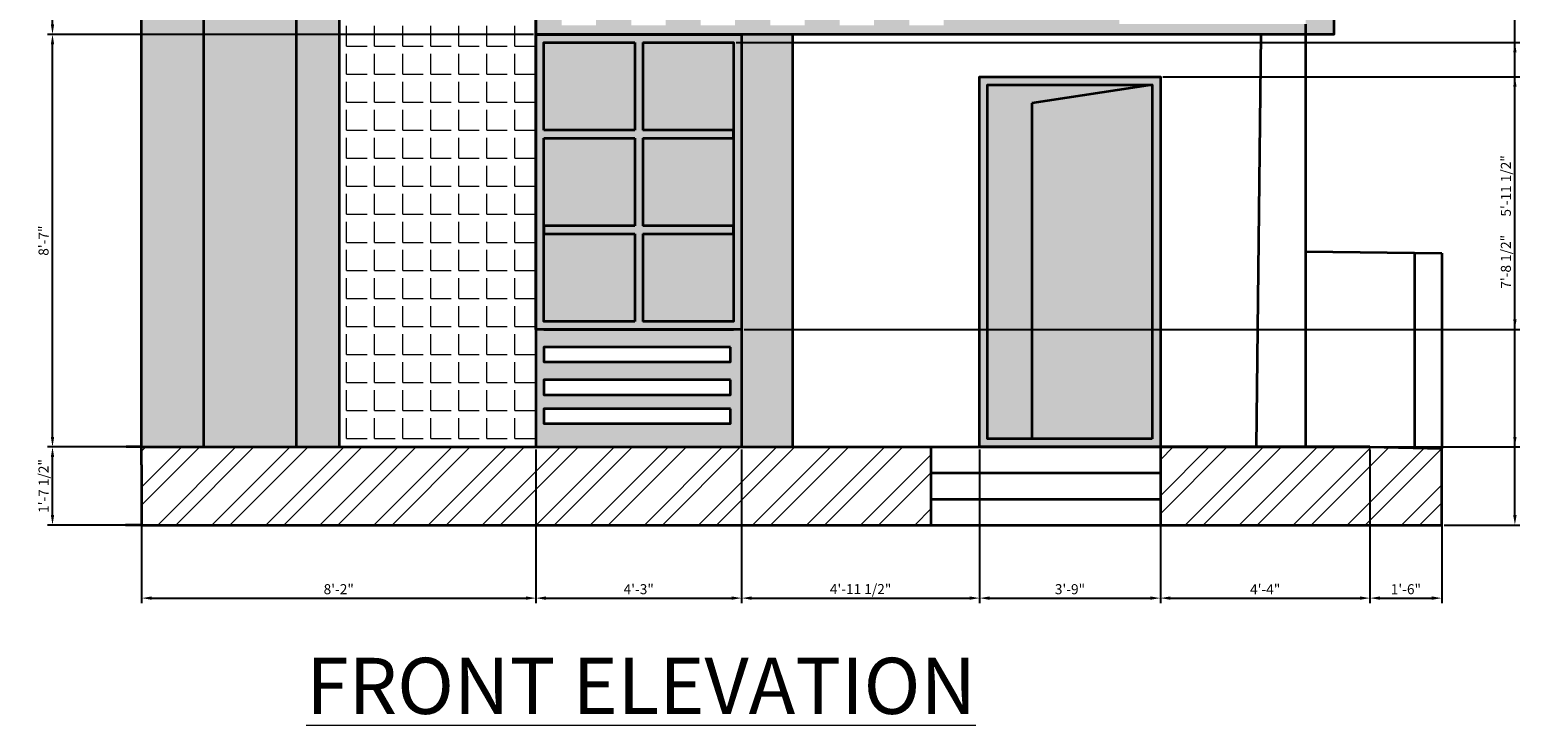
# Model space of a CAD drawing. Units: inches. Extents: x 2117 to 3047, y 1240 to 2266.
# Tile 2 of 4: x 2212 to 2584, y 1884 to 2058. Entities that reach past the tile are written whole.
import ezdxf

# ---------------------------------------------------------------- set-up
doc = ezdxf.new("R2010")
doc.units = ezdxf.units.IN
for name, color, linetype, lineweight in [('A-ANNO-DIMS', 2, 'Continuous', 18), ('A-ANNO-TEXT', 7, 'Continuous', 18), ('A-ELEV', 7, 'Continuous', 35), ('A-ELEV-PATT', 8, 'Continuous', 13)]:
    doc.layers.add(name, color=color, linetype=linetype, lineweight=lineweight)
doc.styles.get("Standard").update_dxf_attribs({"font": 'arial.ttf'})
doc.dimstyles.new('ISO-25', dxfattribs={"dimtxt": 2.5, "dimasz": 2.5, "dimexe": 1.25, "dimexo": 0.625, "dimtad": 1, "dimdec": 1, "dimlunit": 3, "dimtxsty": 'Standard', "dimcen": 2.5, "dimadec": 0, "dimazin": 0, "dimtfac": 1, "dimtdec": 1, "dimtmove": 0, "dimatfit": 3, "dimfxl": 1, "dimarcsym": 0})

# ---------------------------------------------------------------- blocks, each defined once
blk = doc.blocks.new('*D34')
at = {"layer": 'A-ANNO-DIMS', "color": 0, "lineweight": -2, "transparency": 16777216}
for p, q in [((2240.01, 1953.08), (2240.01, 1914.75)), ((2338.23, 1953.08), (2338.23, 1914.75)), ((2242.51, 1916), (2335.73, 1916))]:
    blk.add_line(p, q, dxfattribs=at)
at = {"layer": 'A-ANNO-DIMS', "color": 0, "transparency": 16777216}
for points in [[(2242.51, 1916.42), (2242.51, 1915.58), (2240.01, 1916)], [(2335.73, 1916.42), (2335.73, 1915.58), (2338.23, 1916)]]:
    blk.add_solid(points, dxfattribs=at)
at = {"layer": 'Defpoints', "color": 0, "transparency": 16777216}
for p in [(2240.01, 1953.7), (2338.23, 1953.7), (2338.23, 1916)]:
    blk.add_point(p, dxfattribs=at)
at = {"layer": 'A-ANNO-DIMS', "color": 0, "transparency": 16777216, "insert": (2289.12, 1917.9), "char_height": 2.5, "attachment_point": 5}
blk.add_mtext('8\'-2"', dxfattribs=at)
blk = doc.blocks.new('*D35')
at = {"layer": 'A-ANNO-DIMS', "color": 0, "lineweight": -2, "transparency": 16777216}
for p, q in [((2338.23, 1953.08), (2338.23, 1914.75)), ((2389.48, 1953.08), (2389.48, 1914.75)), ((2340.73, 1916), (2386.98, 1916))]:
    blk.add_line(p, q, dxfattribs=at)
at = {"layer": 'A-ANNO-DIMS', "color": 0, "transparency": 16777216}
for points in [[(2340.73, 1916.42), (2340.73, 1915.58), (2338.23, 1916)], [(2386.98, 1916.42), (2386.98, 1915.58), (2389.48, 1916)]]:
    blk.add_solid(points, dxfattribs=at)
at = {"layer": 'Defpoints', "color": 0, "transparency": 16777216}
for p in [(2338.23, 1953.7), (2389.48, 1953.7), (2389.48, 1916)]:
    blk.add_point(p, dxfattribs=at)
at = {"layer": 'A-ANNO-DIMS', "color": 0, "transparency": 16777216, "insert": (2363.85, 1917.9), "char_height": 2.5, "attachment_point": 5}
blk.add_mtext('4\'-3"', dxfattribs=at)
blk = doc.blocks.new('*D36')
at = {"layer": 'A-ANNO-DIMS', "color": 0, "lineweight": -2, "transparency": 16777216}
for p, q in [((2389.48, 1953.08), (2389.48, 1914.75)), ((2448.76, 1953.08), (2448.76, 1914.75)), ((2391.98, 1916), (2446.26, 1916))]:
    blk.add_line(p, q, dxfattribs=at)
at = {"layer": 'A-ANNO-DIMS', "color": 0, "transparency": 16777216}
for points in [[(2391.98, 1916.42), (2391.98, 1915.58), (2389.48, 1916)], [(2446.26, 1916.42), (2446.26, 1915.58), (2448.76, 1916)]]:
    blk.add_solid(points, dxfattribs=at)
at = {"layer": 'Defpoints', "color": 0, "transparency": 16777216}
for p in [(2389.48, 1953.7), (2448.76, 1953.7), (2448.76, 1916)]:
    blk.add_point(p, dxfattribs=at)
at = {"layer": 'A-ANNO-DIMS', "color": 0, "transparency": 16777216, "insert": (2419.12, 1917.92), "char_height": 2.5, "attachment_point": 5}
blk.add_mtext('4\'-11 1/2"', dxfattribs=at)
blk = doc.blocks.new('*D37')
at = {"layer": 'A-ANNO-DIMS', "color": 0, "lineweight": -2, "transparency": 16777216}
for p, q in [((2448.76, 1953.08), (2448.76, 1914.75)), ((2493.8, 1953.08), (2493.8, 1914.75)), ((2451.26, 1916), (2491.3, 1916))]:
    blk.add_line(p, q, dxfattribs=at)
at = {"layer": 'A-ANNO-DIMS', "color": 0, "transparency": 16777216}
for points in [[(2451.26, 1916.42), (2451.26, 1915.58), (2448.76, 1916)], [(2491.3, 1916.42), (2491.3, 1915.58), (2493.8, 1916)]]:
    blk.add_solid(points, dxfattribs=at)
at = {"layer": 'Defpoints', "color": 0, "transparency": 16777216}
for p in [(2448.76, 1953.7), (2493.8, 1953.7), (2493.8, 1916)]:
    blk.add_point(p, dxfattribs=at)
at = {"layer": 'A-ANNO-DIMS', "color": 0, "transparency": 16777216, "insert": (2471.28, 1917.9), "char_height": 2.5, "attachment_point": 5}
blk.add_mtext('3\'-9"', dxfattribs=at)
blk = doc.blocks.new('*D38')
at = {"layer": 'A-ANNO-DIMS', "color": 0, "lineweight": -2, "transparency": 16777216}
for p, q in [((2493.8, 1953.08), (2493.8, 1914.75)), ((2546.01, 1953.08), (2546.01, 1914.75)), ((2496.3, 1916), (2543.51, 1916))]:
    blk.add_line(p, q, dxfattribs=at)
at = {"layer": 'A-ANNO-DIMS', "color": 0, "transparency": 16777216}
for points in [[(2496.3, 1916.42), (2496.3, 1915.58), (2493.8, 1916)], [(2543.51, 1916.42), (2543.51, 1915.58), (2546.01, 1916)]]:
    blk.add_solid(points, dxfattribs=at)
at = {"layer": 'Defpoints', "color": 0, "transparency": 16777216}
for p in [(2493.8, 1953.7), (2546.01, 1953.7), (2546.01, 1916)]:
    blk.add_point(p, dxfattribs=at)
at = {"layer": 'A-ANNO-DIMS', "color": 0, "transparency": 16777216, "insert": (2519.91, 1917.88), "char_height": 2.5, "attachment_point": 5}
blk.add_mtext('4\'-4"', dxfattribs=at)
blk = doc.blocks.new('*D39')
at = {"layer": 'A-ANNO-DIMS', "color": 0, "lineweight": -2, "transparency": 16777216}
for p, q in [((2546.01, 1953.08), (2546.01, 1914.75)), ((2563.92, 1952.72), (2563.92, 1914.75)), ((2548.51, 1916), (2561.42, 1916))]:
    blk.add_line(p, q, dxfattribs=at)
at = {"layer": 'A-ANNO-DIMS', "color": 0, "transparency": 16777216}
for points in [[(2548.51, 1916.42), (2548.51, 1915.58), (2546.01, 1916)], [(2561.42, 1916.42), (2561.42, 1915.58), (2563.92, 1916)]]:
    blk.add_solid(points, dxfattribs=at)
at = {"layer": 'Defpoints', "color": 0, "transparency": 16777216}
for p in [(2546.01, 1953.7), (2563.92, 1953.34), (2563.92, 1916)]:
    blk.add_point(p, dxfattribs=at)
at = {"layer": 'A-ANNO-DIMS', "color": 0, "transparency": 16777216, "insert": (2554.97, 1917.9), "char_height": 2.5, "attachment_point": 5}
blk.add_mtext('1\'-6"', dxfattribs=at)
blk = doc.blocks.new('*D42')
at = {"layer": 'A-ANNO-DIMS', "color": 0, "lineweight": -2, "transparency": 16777216}
for p, q in [((2239.39, 1953.7), (2216.56, 1953.7)), ((2217.81, 1936.7), (2217.81, 1951.2)), ((2239.39, 1934.2), (2216.56, 1934.2))]:
    blk.add_line(p, q, dxfattribs=at)
at = {"layer": 'A-ANNO-DIMS', "color": 0, "transparency": 16777216}
for points in [[(2217.4, 1951.2), (2218.23, 1951.2), (2217.81, 1953.7)], [(2217.4, 1936.7), (2218.23, 1936.7), (2217.81, 1934.2)]]:
    blk.add_solid(points, dxfattribs=at)
at = {"layer": 'Defpoints', "color": 0, "transparency": 16777216}
for p in [(2217.81, 1953.7), (2240.01, 1953.7), (2240.01, 1934.2)]:
    blk.add_point(p, dxfattribs=at)
at = {"layer": 'A-ANNO-DIMS', "color": 0, "transparency": 16777216, "insert": (2215.9, 1943.95), "char_height": 2.5, "attachment_point": 5, "rotation": 90}
blk.add_mtext('1\'-7 1/2"', dxfattribs=at)
blk = doc.blocks.new('*D43')
at = {"layer": 'A-ANNO-DIMS', "color": 0, "lineweight": -2, "transparency": 16777216}
for p, q in [((2337.6, 2056.54), (2216.56, 2056.54)), ((2217.81, 1956.2), (2217.81, 2054.04)), ((2337.6, 1953.7), (2216.56, 1953.7))]:
    blk.add_line(p, q, dxfattribs=at)
at = {"layer": 'A-ANNO-DIMS', "color": 0, "transparency": 16777216}
for points in [[(2217.4, 2054.04), (2218.23, 2054.04), (2217.81, 2056.54)], [(2217.4, 1956.2), (2218.23, 1956.2), (2217.81, 1953.7)]]:
    blk.add_solid(points, dxfattribs=at)
at = {"layer": 'Defpoints', "color": 0, "transparency": 16777216}
for p in [(2217.81, 2056.54), (2338.23, 2056.54), (2338.23, 1953.7)]:
    blk.add_point(p, dxfattribs=at)
at = {"layer": 'A-ANNO-DIMS', "color": 0, "transparency": 16777216, "insert": (2215.91, 2005.12), "char_height": 2.5, "attachment_point": 5, "rotation": 90}
blk.add_mtext('8\'-7"', dxfattribs=at)
blk = doc.blocks.new('*D44')
at = {"layer": 'A-ANNO-DIMS', "color": 0, "lineweight": -2, "transparency": 16777216}
for p, q in [((2337.6, 2079.7), (2216.56, 2079.7)), ((2217.81, 2059.04), (2217.81, 2077.2)), ((2337.6, 2056.54), (2216.56, 2056.54))]:
    blk.add_line(p, q, dxfattribs=at)
at = {"layer": 'A-ANNO-DIMS', "color": 0, "transparency": 16777216}
for points in [[(2217.4, 2077.2), (2218.23, 2077.2), (2217.81, 2079.7)], [(2217.4, 2059.04), (2218.23, 2059.04), (2217.81, 2056.54)]]:
    blk.add_solid(points, dxfattribs=at)
at = {"layer": 'Defpoints', "color": 0, "transparency": 16777216}
for p in [(2217.81, 2079.7), (2338.23, 2079.7), (2338.23, 2056.54)]:
    blk.add_point(p, dxfattribs=at)
at = {"layer": 'A-ANNO-DIMS', "color": 0, "transparency": 16777216, "insert": (2215.93, 2068.12), "char_height": 2.5, "attachment_point": 5, "rotation": 90}
blk.add_mtext('1\'-11"', dxfattribs=at)
blk = doc.blocks.new('*D48')
at = {"layer": 'A-ANNO-DIMS', "color": 0, "lineweight": -2, "transparency": 16777216}
for p, q in [((2546.64, 2241.7), (2583.37, 2241.7)), ((2582.12, 1936.7), (2582.12, 2239.2)), ((2564.54, 1934.2), (2583.37, 1934.2))]:
    blk.add_line(p, q, dxfattribs=at)
at = {"layer": 'A-ANNO-DIMS', "color": 0, "transparency": 16777216}
for points in [[(2581.7, 2239.2), (2582.54, 2239.2), (2582.12, 2241.7)], [(2581.7, 1936.7), (2582.54, 1936.7), (2582.12, 1934.2)]]:
    blk.add_solid(points, dxfattribs=at)
at = {"layer": 'Defpoints', "color": 0, "transparency": 16777216}
for p in [(2546.01, 2241.7), (2582.12, 2241.7), (2563.92, 1934.2)]:
    blk.add_point(p, dxfattribs=at)
at = {"layer": 'A-ANNO-DIMS', "color": 0, "transparency": 16777216, "insert": (2580.2, 2087.95), "char_height": 2.5, "attachment_point": 5, "rotation": 90}
blk.add_mtext('25\'-7 1/2"', dxfattribs=at)
blk = doc.blocks.new('*D49')
at = {"layer": 'A-ANNO-DIMS', "color": 0, "lineweight": -2, "transparency": 16777216}
for p, q in [((2494.42, 2046), (2583.37, 2046)), ((2582.12, 1956.2), (2582.12, 2043.5)), ((2494.42, 1953.7), (2583.37, 1953.7))]:
    blk.add_line(p, q, dxfattribs=at)
at = {"layer": 'A-ANNO-DIMS', "color": 0, "transparency": 16777216}
for points in [[(2581.7, 2043.5), (2582.54, 2043.5), (2582.12, 2046)], [(2581.7, 1956.2), (2582.54, 1956.2), (2582.12, 1953.7)]]:
    blk.add_solid(points, dxfattribs=at)
at = {"layer": 'Defpoints', "color": 0, "transparency": 16777216}
for p in [(2493.8, 2046), (2582.12, 2046), (2493.8, 1953.7)]:
    blk.add_point(p, dxfattribs=at)
at = {"layer": 'A-ANNO-DIMS', "color": 0, "transparency": 16777216, "insert": (2580.2, 1999.85), "char_height": 2.5, "attachment_point": 5, "rotation": 90}
blk.add_mtext('7\'-8 1/2"', dxfattribs=at)
blk = doc.blocks.new('*D52')
at = {"layer": 'A-ANNO-DIMS', "color": 0, "lineweight": -2, "transparency": 16777216}
for p, q in [((2388.1, 2054.54), (2583.37, 2054.54)), ((2582.12, 1985.49), (2582.12, 2052.04)), ((2390.1, 1982.99), (2583.37, 1982.99))]:
    blk.add_line(p, q, dxfattribs=at)
at = {"layer": 'A-ANNO-DIMS', "color": 0, "transparency": 16777216}
for points in [[(2581.7, 2052.04), (2582.54, 2052.04), (2582.12, 2054.54)], [(2581.7, 1985.49), (2582.54, 1985.49), (2582.12, 1982.99)]]:
    blk.add_solid(points, dxfattribs=at)
at = {"layer": 'Defpoints', "color": 0, "transparency": 16777216}
for p in [(2387.48, 2054.54), (2582.12, 2054.54), (2389.48, 1982.99)]:
    blk.add_point(p, dxfattribs=at)
at = {"layer": 'A-ANNO-DIMS', "color": 0, "transparency": 16777216, "insert": (2580.2, 2018.77), "char_height": 2.5, "attachment_point": 5, "rotation": 90}
blk.add_mtext('5\'-11 1/2"', dxfattribs=at)

msp = doc.modelspace()

# ---------------------------------------------------------------- hatches: boundary and pattern name
at = {"layer": 'A-ELEV-PATT'}
h = msp.add_hatch(dxfattribs=at)
h.set_pattern_fill('AR-CONC', color=256, scale=30)
h.set_pattern_definition([(50, (-387, -0.0008), (5465.5, -478), [571.5, -6286.5]), (355, (-387, -0.0008), (-1057.3, 5731.7), [457.2, -5029.2]), (100.45, (68.6, -40), (4408, 5253.5), [485.7, -5342.7]), (46.18, (-387, 1524), (8132.4, -1261), [857.2, -9429.8]), (96.64, (291, 1419), (7122, 7423), [728.6, -8014]), (351.18, (-387, 1524), (7122, 7423), [686, -7544]), (21, (375, 1143), (4548.4, -3068), [571.5, -6286.5]), (326, (375, 1143), (1854, 5525.6), [457.2, -5029.2]), (71.45, (754, 887.3), (6402.5, 2457.7), [485.7, -5342.7]), (37.5, (-386.8, -0.0008), (92.7, 2536.7), [0, -4968.24, 0, -5105.4, 0, -5048.25]), (7.5, (-386.8, -0.0008), (2004.6, 3005.4), [0, -2910.84, 0, -4853.94, 0, -1924.05]), (327.5, (-2086.1, -0.0008), (4067.7, -171.9), [0, -1905, 0, -5943.6, 0, -7886.7]), (317.5, (-2848, -0.0008), (4443.9, 762.8), [0, -2476.5, 0, -3947.2, 0, -5600.7])])
h.paths.add_polyline_path([(2249.02, 2199.7), (2537.02, 2199.7), (2537.02, 2175.7), (2546.02, 2175.7), (2546.02, 2205.7), (2240.02, 2205.7), (2240.02, 2175.7), (2249.02, 2175.7)])
h.paths.add_polyline_path([(2546.02, 2079.7), (2240.02, 2079.7), (2240.02, 2049.7), (2249.02, 2049.7), (2249.02, 2073.7), (2537.02, 2073.7), (2537.02, 2049.7), (2546.02, 2049.7)])
h = msp.add_hatch(color=256, dxfattribs=at)
h.dxf.hatch_style = 1
h.paths.add_polyline_path([(2537.01, 2199.7), (2240.01, 2199.7), (2240.01, 1953.7), (2255.43, 1953.7), (2255.43, 2181.7), (2537.01, 2181.7)])
h = msp.add_hatch(color=256, dxfattribs=at)
h.dxf.hatch_style = 1
h.paths.add_polyline_path([(2278.52, 2168.93), (2402.12, 2168.93), (2402.12, 2181.7), (2255.43, 2181.7), (2255.43, 2079.7), (2278.52, 2079.7)])
h.paths.add_polyline_path([(2278.52, 2079.7), (2255.43, 2079.7), (2255.43, 2073.7), (2278.52, 2073.7)])
h.paths.add_polyline_path([(2278.52, 2073.7), (2255.43, 2073.7), (2255.43, 1953.7), (2278.52, 1953.7)])
h = msp.add_hatch(color=256, dxfattribs=at)
h.dxf.hatch_style = 1
h.paths.add_polyline_path([(2289.19, 2160.2), (2405.83, 2160.2), (2405.83, 2168.93), (2402.12, 2168.93), (2278.52, 2168.93), (2278.52, 1953.7), (2289.19, 1953.7)])
h = msp.add_hatch(dxfattribs=at)
h.set_pattern_fill('ANGLE', color=256)
h.set_pattern_definition([(0, (0, 0), (0, 6.985), [5.08, -1.905]), (90, (0, 0), (-6.985, 4e-16), [5.08, -1.905])])
h.paths.add_polyline_path([(2338.23, 2160.2), (2289.19, 2160.2), (2289.19, 1953.7), (2338.23, 1953.7)])
h = msp.add_hatch(color=256, dxfattribs=at)
h.dxf.hatch_style = 1
h.paths.add_polyline_path([(2338.23, 2079.7), (2338.23, 2056.54), (2537.01, 2056.54), (2537.01, 2079.7), (2535.26, 2079.7), (2535.26, 2061), (2532.24, 2061), (2532.24, 2079.7)])
h.paths.add_polyline_path([(2529.98, 2077.15), (2529.98, 2073.48), (2483.54, 2073.48), (2483.54, 2077.15)], flags=16)
h.paths.add_polyline_path([(2529.98, 2069.97), (2529.98, 2066.3), (2483.54, 2066.3), (2483.54, 2069.97)], flags=16)
h.paths.add_polyline_path([(2529.98, 2062.78), (2529.98, 2059.12), (2483.54, 2059.12), (2483.54, 2062.78)], flags=16)
h.paths.add_polyline_path([(2439.81, 2077.77), (2439.81, 2058.82), (2431.24, 2058.82), (2431.24, 2077.77)], flags=16)
h.paths.add_polyline_path([(2422.49, 2077.77), (2422.49, 2058.82), (2413.92, 2058.82), (2413.92, 2077.77)], flags=16)
h.paths.add_polyline_path([(2405.18, 2077.77), (2405.18, 2058.82), (2396.61, 2058.82), (2396.61, 2077.77)], flags=16)
h.paths.add_polyline_path([(2387.86, 2077.77), (2387.86, 2058.82), (2379.29, 2058.82), (2379.29, 2077.77)], flags=16)
h.paths.add_polyline_path([(2370.54, 2077.77), (2370.54, 2058.82), (2361.97, 2058.82), (2361.97, 2077.77)], flags=16)
h.paths.add_polyline_path([(2353.23, 2077.77), (2353.23, 2058.82), (2344.66, 2058.82), (2344.66, 2077.77)], flags=16)
h = msp.add_hatch(color=256, dxfattribs=at)
h.dxf.hatch_style = 1
h.paths.add_polyline_path([(2387.48, 2056.54), (2340.23, 2056.54), (2340.23, 2054.54), (2387.48, 2054.54)], flags=17)
h.paths.add_polyline_path([(2389.48, 2056.54), (2387.48, 2056.54), (2387.48, 2054.54), (2387.48, 1984.99), (2340.23, 1984.99), (2340.23, 2054.54), (2340.23, 2056.54), (2338.23, 2056.54), (2338.23, 1982.99), (2389.48, 1982.99)])
h.paths.add_polyline_path([(2364.85, 2008.84), (2362.85, 2008.84), (2362.85, 2006.84), (2364.85, 2006.84)], flags=17)
h.paths.add_polyline_path([(2387.48, 2008.84), (2364.85, 2008.84), (2364.85, 2006.84), (2387.48, 2006.84)], flags=17)
h.paths.add_polyline_path([(2362.85, 2008.84), (2340.23, 2008.84), (2340.23, 2006.84), (2362.85, 2006.84)], flags=17)
h.paths.add_polyline_path([(2364.85, 2030.69), (2362.85, 2030.69), (2362.85, 2008.84), (2364.85, 2008.84)], flags=17)
h.paths.add_polyline_path([(2364.85, 2006.84), (2362.85, 2006.84), (2362.85, 1984.99), (2364.85, 1984.99)], flags=17)
h.paths.add_polyline_path([(2364.85, 2054.54), (2362.85, 2054.54), (2362.85, 2032.69), (2364.85, 2032.69)], flags=17)
h.paths.add_polyline_path([(2364.85, 2032.69), (2362.85, 2032.69), (2362.85, 2030.69), (2364.85, 2030.69)], flags=17)
h.paths.add_polyline_path([(2362.85, 2032.69), (2340.23, 2032.69), (2340.23, 2030.69), (2362.85, 2030.69)], flags=17)
h.paths.add_polyline_path([(2387.48, 2032.69), (2364.85, 2032.69), (2364.85, 2030.69), (2387.48, 2030.69)], flags=17)
h = msp.add_hatch(color=256, dxfattribs=at)
h.dxf.hatch_style = 1
h.paths.add_polyline_path([(2402.12, 2056.54), (2389.48, 2056.54), (2389.48, 1982.99), (2389.48, 1953.7), (2402.12, 1953.7)])
h = msp.add_hatch(color=256, dxfattribs=at)
h.dxf.hatch_style = 1
h.paths.add_polyline_path([(2387.48, 2054.54), (2364.85, 2054.54), (2364.85, 2032.69), (2387.48, 2032.69)])
h.paths.add_polyline_path([(2387.48, 2030.69), (2364.85, 2030.69), (2364.85, 2008.84), (2387.48, 2008.84)])
h.paths.add_polyline_path([(2387.48, 2006.84), (2364.85, 2006.84), (2364.85, 1984.99), (2387.48, 1984.99)])
h.paths.add_polyline_path([(2362.85, 2006.84), (2340.23, 2006.84), (2340.23, 1984.99), (2362.85, 1984.99)])
h.paths.add_polyline_path([(2362.85, 2030.69), (2340.23, 2030.69), (2340.23, 2008.84), (2362.85, 2008.84)])
h.paths.add_polyline_path([(2362.85, 2054.54), (2340.23, 2054.54), (2340.23, 2032.69), (2362.85, 2032.69)])
h = msp.add_hatch(color=256, dxfattribs=at)
h.dxf.hatch_style = 1
h.paths.add_polyline_path([(2493.8, 2046), (2448.76, 2046), (2448.76, 1953.7), (2493.8, 1953.7)])
h.paths.add_polyline_path([(2491.8, 2044), (2491.8, 1955.7), (2450.76, 1955.7), (2450.76, 2044)], flags=16)
h.paths.add_polyline_path([(2491.8, 2044), (2461.79, 2039.39), (2461.79, 1955.7), (2491.8, 1955.7)], flags=0)
h = msp.add_hatch(color=256, dxfattribs=at)
h.dxf.hatch_style = 1
h.paths.add_polyline_path([(2461.79, 2039.39), (2491.8, 2044), (2450.76, 2044), (2450.76, 1955.7), (2461.79, 1955.7)])
h = msp.add_hatch(color=256, dxfattribs=at)
h.dxf.hatch_style = 1
h.paths.add_polyline_path([(2491.8, 2044), (2461.79, 2039.39), (2461.79, 1955.7), (2491.8, 1955.7)])
h = msp.add_hatch(color=256, dxfattribs=at)
h.dxf.hatch_style = 1
h.paths.add_polyline_path([(2389.48, 1982.99), (2338.23, 1982.99), (2338.23, 1953.7), (2389.48, 1953.7)])
h.paths.add_polyline_path([(2340.25, 1974.89), (2340.25, 1978.56), (2386.69, 1978.56), (2386.69, 1974.89)], flags=16)
h.paths.add_polyline_path([(2386.69, 1970.38), (2386.69, 1966.71), (2340.25, 1966.71), (2340.25, 1970.38)], flags=16)
h.paths.add_polyline_path([(2386.69, 1963.19), (2386.69, 1959.52), (2340.25, 1959.52), (2340.25, 1963.19)], flags=16)
h = msp.add_hatch(dxfattribs=at)
h.set_pattern_fill('AR-CONC', color=256, scale=30)
h.set_pattern_definition([(50, (-387, 0), (5465.5, -478), [571.5, -6286.5]), (355, (-387, 0), (-1057.3, 5731.7), [457.2, -5029.2]), (100.45, (68.6, -40), (4408, 5253.5), [485.7, -5342.7]), (46.18, (-387, 1524), (8132.4, -1261), [857.2, -9429.8]), (96.64, (291, 1419), (7122, 7423), [728.6, -8014]), (351.18, (-387, 1524), (7122, 7423), [686, -7544]), (21, (375, 1143), (4548.4, -3068), [571.5, -6286.5]), (326, (375, 1143), (1854, 5525.6), [457.2, -5029.2]), (71.45, (754, 887.3), (6402.5, 2457.7), [485.7, -5342.7]), (37.5, (-386.8, 0), (92.7, 2536.7), [0, -4968.24, 0, -5105.4, 0, -5048.25]), (7.5, (-386.8, 0), (2004.6, 3005.4), [0, -2910.84, 0, -4853.94, 0, -1924.05]), (327.5, (-2086.1, 0), (4067.7, -171.9), [0, -1905, 0, -5943.6, 0, -7886.7]), (317.5, (-2848, 0), (4443.9, 762.8), [0, -2476.5, 0, -3947.2, 0, -5600.7])])
h.paths.add_polyline_path([(2546.01, 1953.7), (2240.01, 1953.7), (2240.01, 1949.2), (2546.01, 1949.2)])
h = msp.add_hatch(dxfattribs=at)
h.set_pattern_fill('ANSI32', color=256)
h.paths.add_polyline_path([(2436.73, 1953.7), (2240.01, 1953.7), (2240.01, 1949.2), (2240.01, 1934.2), (2436.73, 1934.2)])
h.paths.add_polyline_path([(2563.92, 1953.34), (2546.01, 1953.7), (2493.8, 1953.7), (2493.8, 1934.2), (2546.01, 1934.2), (2550.01, 1934.2), (2563.92, 1934.2)])

# ---------------------------------------------------------------- linework, layer by layer
at = {"layer": 'A-ELEV'}
for p, q in [((2240.01, 1949.2), (2240.01, 2241.7)), ((2255.43, 2181.7), (2255.43, 1953.7)), ((2278.52, 2168.93), (2278.52, 1953.7)), ((2289.19, 2160.2), (2289.19, 1953.7)), ((2338.23, 2160.2), (2338.23, 1953.7)), ((2402.12, 2056.54), (2402.12, 1953.7)), ((2518.83, 2056.54), (2517.63, 1953.7)), ((2529.98, 2059.12), (2529.98, 1953.7)), ((2362.85, 2054.54), (2362.85, 2032.69)), ((2364.85, 2054.54), (2364.85, 2032.69)), ((2491.8, 2044), (2461.79, 2039.39)), ((2461.79, 2039.39), (2461.79, 1955.7)), ((2362.85, 2030.69), (2362.85, 2008.84)), ((2364.85, 2030.69), (2364.85, 2008.84)), ((2362.85, 2006.84), (2362.85, 1984.99)), ((2364.85, 2006.84), (2364.85, 1984.99)), ((2529.98, 2002.38), (2563.92, 2001.98)), ((2557.14, 2001.98), (2557.14, 1953.34)), ((2563.92, 2001.98), (2563.92, 1953.34)), ((2389.48, 1982.99), (2389.48, 1953.7)), ((2240.01, 1953.7), (2236.2, 1953.7)), ((2240.01, 1953.7), (2546.01, 1953.7)), ((2436.73, 1934.2), (2436.73, 1953.7)), ((2436.73, 1953.7), (2493.8, 1953.7)), ((2436.73, 1953.7), (2436.73, 1953.7)), ((2436.73, 1953.7), (2436.73, 1953.7)), ((2436.73, 1953.7), (2493.8, 1953.7)), ((2436.73, 1953.7), (2493.8, 1953.7)), ((2436.73, 1953.7), (2493.8, 1953.7)), ((2436.73, 1953.7), (2493.8, 1953.7)), ((2493.8, 1953.7), (2493.8, 1953.7)), ((2546.01, 1953.7), (2493.8, 1953.7)), ((2493.8, 1953.7), (2493.8, 1934.2)), ((2546.01, 1953.7), (2563.92, 1953.34)), ((2563.92, 1934.2), (2563.92, 1953.34)), ((2240.01, 1949.2), (2240.01, 1934.2)), ((2436.73, 1947.2), (2493.8, 1947.2)), ((2436.73, 1940.7), (2493.8, 1940.7)), ((2240.01, 1934.2), (2236.01, 1934.2)), ((2240.01, 1934.2), (2534.01, 1934.2)), ((2393.06, 1934.2), (2546.01, 1934.2)), ((2436.73, 1934.2), (2493.8, 1934.2)), ((2436.73, 1934.2), (2493.8, 1934.2)), ((2546.01, 1934.2), (2550.01, 1934.2)), ((2550.01, 1934.2), (2563.92, 1934.2))]:
    msp.add_line(p, q, dxfattribs=at)
for points in [[(2537.01, 2079.7), (2537.01, 2056.54), (2338.23, 2056.54), (2338.23, 2079.7), (2507.01, 2079.7)], [(2387.48, 2056.54), (2340.23, 2056.54)], [(2340.23, 2054.54), (2362.85, 2054.54)], [(2340.23, 2032.69), (2340.23, 2054.54), (2362.85, 2054.54)], [(2364.85, 2054.54), (2387.48, 2054.54), (2387.48, 1984.99), (2364.85, 1984.99)], [(2364.85, 2054.54), (2387.48, 2054.54)], [(2362.85, 2032.69), (2340.23, 2032.69)], [(2340.23, 2030.69), (2362.85, 2030.69)], [(2362.85, 1984.99), (2340.23, 1984.99), (2340.23, 2030.69)], [(2364.85, 2030.69), (2387.48, 2030.69), (2387.48, 2032.69), (2364.85, 2032.69)], [(2362.85, 2008.84), (2340.23, 2008.84), (2340.23, 2006.84), (2362.85, 2006.84)], [(2364.85, 2006.84), (2387.48, 2006.84), (2387.48, 2008.84), (2364.85, 2008.84)], [(2362.85, 1984.99), (2340.23, 1984.99)], [(2340.23, 1982.99), (2387.48, 1982.99)], [(2387.48, 1984.99), (2364.85, 1984.99)]]:
    msp.add_lwpolyline(points, dxfattribs=at)
for points in [[(2338.23, 2056.54), (2389.48, 2056.54), (2389.48, 1982.99), (2338.23, 1982.99)], [(2493.8, 1953.7), (2448.76, 1953.7), (2448.76, 2046), (2493.8, 2046)], [(2491.8, 1955.7), (2450.76, 1955.7), (2450.76, 2044), (2491.8, 2044)], [(2386.69, 1978.56), (2340.25, 1978.56), (2340.25, 1974.89), (2386.69, 1974.89)], [(2386.69, 1970.38), (2340.25, 1970.38), (2340.25, 1966.71), (2386.69, 1966.71)], [(2386.69, 1963.19), (2340.25, 1963.19), (2340.25, 1959.52), (2386.69, 1959.52)]]:
    msp.add_lwpolyline(points, close=True, dxfattribs=at)

# ---------------------------------------------------------------- texts
at = {"layer": 'A-ANNO-TEXT', "insert": (2281, 1901.12), "char_height": 14, "attachment_point": 1}
msp.add_mtext_dynamic_manual_height_columns('{\\LFRONT ELEVATION}', width=221.8965, gutter_width=70, heights=[0], dxfattribs=at)

# ---------------------------------------------------------------- dimensions: what is measured, and where the dimension line sits
at = {"layer": 'A-ANNO-DIMS'}
for base, p1, p2, picture, middle in [((2582.12, 2241.7), (2563.92, 1934.2), (2546.01, 2241.7), '*D48', (2580.2, 2087.95)), ((2217.81, 2079.7), (2338.23, 2056.54), (2338.23, 2079.7), '*D44', (2215.93, 2068.12)), ((2217.81, 2056.54), (2338.23, 1953.7), (2338.23, 2056.54), '*D43', (2215.91, 2005.12)), ((2582.1185, 2054.5432), (2389.4771, 1982.9947), (2387.4771, 2054.5432), '*D52', (2580.2009, 2018.769)), ((2582.12, 2046), (2493.8, 1953.7), (2493.8, 2046), '*D49', (2580.2, 1999.85)), ((2217.81, 1953.7), (2240.01, 1934.2), (2240.01, 1953.7), '*D42', (2215.9, 1943.95))]:
    dim = msp.add_linear_dim(base=base, p1=p1, p2=p2, angle=90, dimstyle='ISO-25', override={"dimdec": 1, "dimlfac": 1, "dimrnd": 0, "dimzin": 1, "dimdsep": 46, "dimlunit": 4, "dimfrac": 2}, dxfattribs=at)
    dim.commit()
    dim.dimension.update_dxf_attribs({"geometry": picture, "text_midpoint": middle})
for base, p1, p2, picture, middle in [((2338.23, 1916), (2240.01, 1953.7), (2338.23, 1953.7), '*D34', (2289.12, 1917.9)), ((2389.4771, 1916.0008), (2338.2278, 1953.7008), (2389.4771, 1953.7008), '*D35', (2363.8525, 1917.9031)), ((2448.76, 1916), (2389.48, 1953.7), (2448.76, 1953.7), '*D36', (2419.12, 1917.92)), ((2493.8, 1916), (2448.76, 1953.7), (2493.8, 1953.7), '*D37', (2471.28, 1917.9)), ((2546.01, 1916), (2493.8, 1953.7), (2546.01, 1953.7), '*D38', (2519.91, 1917.88)), ((2563.92, 1916), (2546.01, 1953.7), (2563.92, 1953.34), '*D39', (2554.97, 1917.9))]:
    dim = msp.add_linear_dim(base=base, p1=p1, p2=p2, dimstyle='ISO-25', override={"dimdec": 1, "dimlfac": 1, "dimrnd": 0, "dimzin": 1, "dimdsep": 46, "dimlunit": 4, "dimfrac": 2}, dxfattribs=at)
    dim.commit()
    dim.dimension.update_dxf_attribs({"geometry": picture, "text_midpoint": middle})

doc.saveas('drawing.dxf')
